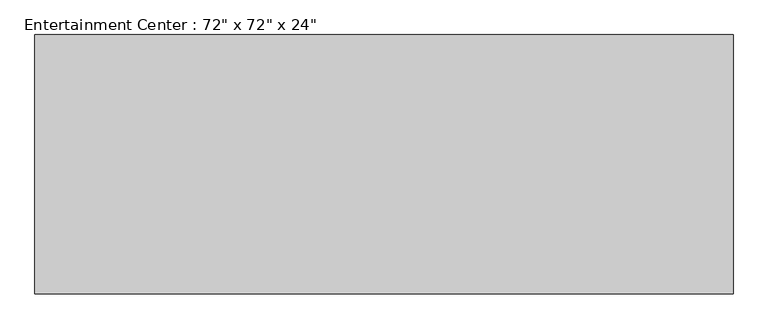
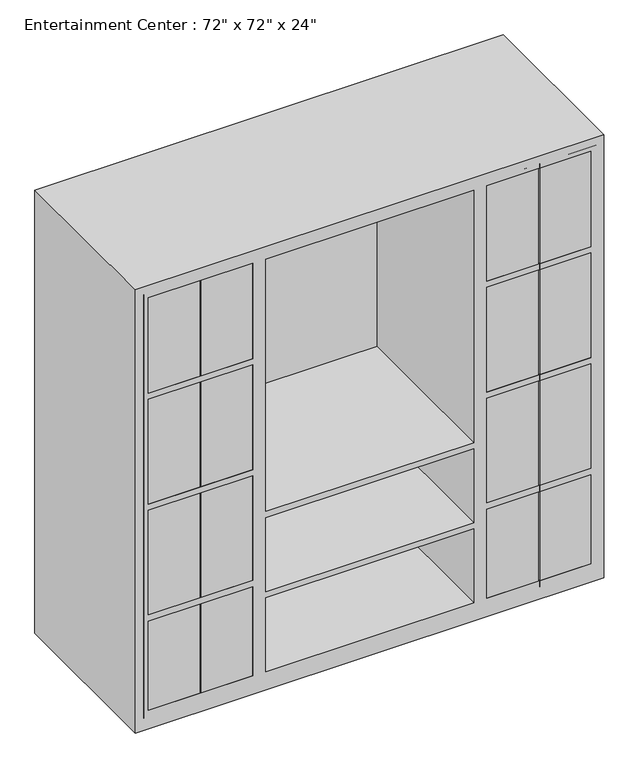
"""IFC4 building model written with IfcOpenShell, lengths in millimetres: furniture geometry."""

from ifc_helpers import new_model, si_unit, point, frame, frame_2d, origin, place, context, project, spatial, polyline, circle_curve, trimmed, segment, composite_curve, outline, extrude, faceted_brep, source, transform, mapped, element, save


def furniture_cf0b6580(model_context):
    return source(origin(), model_context, "Body", "SolidModel", [
        faceted_brep([(914.4, -781.05, 0.0), (914.4, -781.05, 1828.8), (-914.4, -781.05, 1828.8), (-914.4, -781.05, 0.0), (-457.2, -781.05, 1778.0), (-457.2, -781.05, 1384.3), (-863.6, -781.05, 1384.3), (-863.6, -781.05, 1778.0), (-457.2, -781.05, 76.2), (-863.6, -781.05, 76.2), (-863.6, -781.05, 444.5), (-457.2, -781.05, 444.5), (863.6, -781.05, 1384.3), (457.2, -781.05, 1384.3), (457.2, -781.05, 1778.0), (863.6, -781.05, 1778.0), (-406.4, -781.05, 736.6), (-406.4, -781.05, 1778.0), (406.4, -781.05, 1778.0), (406.4, -781.05, 736.6), (406.4, -781.05, 76.2), (-406.4, -781.05, 76.2), (-406.4, -781.05, 381.0), (406.4, -781.05, 381.0), (863.6, -781.05, 76.2), (457.2, -781.05, 76.2), (457.2, -781.05, 444.5), (863.6, -781.05, 444.5), (-863.6, -781.05, 469.9), (-863.6, -781.05, 901.7), (-457.2, -781.05, 901.7), (-457.2, -781.05, 469.9), (-457.2, -781.05, 1358.9), (-457.2, -781.05, 927.1), (-863.6, -781.05, 927.1), (-863.6, -781.05, 1358.9), (457.2, -781.05, 1358.9), (863.6, -781.05, 1358.9), (863.6, -781.05, 927.1), (457.2, -781.05, 927.1), (457.2, -781.05, 901.7), (863.6, -781.05, 901.7), (863.6, -781.05, 469.9), (457.2, -781.05, 469.9), (406.4, -781.05, 406.4), (-406.4, -781.05, 406.4), (-406.4, -781.05, 711.2), (406.4, -781.05, 711.2), (914.4, -101.6, 0.0), (-914.4, -101.6, 0.0), (-914.4, -101.6, 1828.8), (914.4, -101.6, 1828.8), (-457.2, -127.0, 1778.0), (-457.2, -127.0, 1384.3), (-863.6, -127.0, 1384.3), (-863.6, -127.0, 1778.0), (-457.2, -127.0, 76.2), (-863.6, -127.0, 76.2), (-863.6, -127.0, 444.5), (-457.2, -127.0, 444.5), (863.6, -127.0, 1384.3), (457.2, -127.0, 1384.3), (457.2, -127.0, 1778.0), (863.6, -127.0, 1778.0), (-406.4, -127.0, 736.6), (-406.4, -127.0, 1778.0), (406.4, -127.0, 1778.0), (406.4, -127.0, 736.6), (406.4, -127.0, 76.2), (-406.4, -127.0, 76.2), (-406.4, -127.0, 381.0), (406.4, -127.0, 381.0), (863.6, -127.0, 76.2), (457.2, -127.0, 76.2), (457.2, -127.0, 444.5), (863.6, -127.0, 444.5), (-863.6, -127.0, 469.9), (-863.6, -127.0, 901.7), (-457.2, -127.0, 901.7), (-457.2, -127.0, 469.9), (-457.2, -127.0, 1358.9), (-457.2, -127.0, 927.1), (-863.6, -127.0, 927.1), (-863.6, -127.0, 1358.9), (457.2, -127.0, 1358.9), (863.6, -127.0, 1358.9), (863.6, -127.0, 927.1), (457.2, -127.0, 927.1), (457.2, -127.0, 901.7), (863.6, -127.0, 901.7), (863.6, -127.0, 469.9), (457.2, -127.0, 469.9), (406.4, -127.0, 406.4), (-406.4, -127.0, 406.4), (-406.4, -127.0, 711.2), (406.4, -127.0, 711.2)], [[[0, 1, 2, 3], [4, 5, 6, 7], [8, 9, 10, 11], [12, 13, 14, 15], [16, 17, 18, 19], [20, 21, 22, 23], [24, 25, 26, 27], [28, 29, 30, 31], [32, 33, 34, 35], [36, 37, 38, 39], [40, 41, 42, 43], [44, 45, 46, 47]], [[48, 49, 50, 51]], [[1, 0, 48, 51]], [[2, 1, 51, 50]], [[3, 2, 50, 49]], [[0, 3, 49, 48]], [[5, 4, 52, 53]], [[6, 5, 53, 54]], [[7, 6, 54, 55]], [[4, 7, 55, 52]], [[9, 8, 56, 57]], [[10, 9, 57, 58]], [[11, 10, 58, 59]], [[8, 11, 59, 56]], [[13, 12, 60, 61]], [[14, 13, 61, 62]], [[15, 14, 62, 63]], [[12, 15, 63, 60]], [[17, 16, 64, 65]], [[18, 17, 65, 66]], [[19, 18, 66, 67]], [[16, 19, 67, 64]], [[21, 20, 68, 69]], [[22, 21, 69, 70]], [[23, 22, 70, 71]], [[20, 23, 71, 68]], [[25, 24, 72, 73]], [[26, 25, 73, 74]], [[27, 26, 74, 75]], [[24, 27, 75, 72]], [[29, 28, 76, 77]], [[30, 29, 77, 78]], [[31, 30, 78, 79]], [[28, 31, 79, 76]], [[33, 32, 80, 81]], [[34, 33, 81, 82]], [[35, 34, 82, 83]], [[32, 35, 83, 80]], [[37, 36, 84, 85]], [[38, 37, 85, 86]], [[39, 38, 86, 87]], [[36, 39, 87, 84]], [[41, 40, 88, 89]], [[42, 41, 89, 90]], [[43, 42, 90, 91]], [[40, 43, 91, 88]], [[45, 44, 92, 93]], [[46, 45, 93, 94]], [[47, 46, 94, 95]], [[44, 47, 95, 92]], [[53, 52, 55, 54]], [[57, 56, 59, 58]], [[61, 60, 63, 62]], [[65, 64, 67, 66]], [[69, 68, 71, 70]], [[73, 72, 75, 74]], [[77, 76, 79, 78]], [[81, 80, 83, 82]], [[85, 84, 87, 86]], [[89, 88, 91, 90]], [[93, 92, 95, 94]]]),
        extrude(outline(composite_curve([segment(polyline([(1003.3, -632.9986452), (1003.3, -657.225), (825.5, -657.225), (825.5, -632.9986452)]), True, "CONTINUOUS"), segment(trimmed(circle_curve(frame_2d((850.9, -632.9986452)), 25.4), [point((825.5, -632.9986452))], [point((850.9, -607.5986452))], False, "CARTESIAN"), True, "CONTINUOUS"), segment(polyline([(850.9, -607.5986452), (977.9, -607.5986452)]), True, "CONTINUOUS"), segment(trimmed(circle_curve(frame_2d((977.9, -632.9986452)), 25.4), [point((977.9, -607.5986452))], [point((1003.3, -632.9986452))], False, "CARTESIAN"), True, "CONTINUOUS")], self_intersect=False)), frame((0.0, -714.375, 0.0), z_axis=(0.0, 1.0, 0.0), x_axis=(0.0, 0.0, 1.0)), (0.0, 0.0, 1.0), 3.175),
        extrude(outline(composite_curve([segment(trimmed(circle_curve(frame_2d((977.9, -688.18125)), 25.4), [point((1003.3, -688.18125))], [point((977.9, -713.58125))], False, "CARTESIAN"), True, "CONTINUOUS"), segment(polyline([(977.9, -713.58125), (850.9, -713.58125)]), True, "CONTINUOUS"), segment(trimmed(circle_curve(frame_2d((850.9, -688.18125)), 25.4), [point((850.9, -713.58125))], [point((825.5, -688.18125))], False, "CARTESIAN"), True, "CONTINUOUS"), segment(polyline([(825.5, -688.18125), (825.5, -663.575), (1003.3, -663.575), (1003.3, -688.18125)]), True, "CONTINUOUS")], self_intersect=False)), frame((0.0, -714.375, 0.0), z_axis=(0.0, 1.0, 0.0), x_axis=(0.0, 0.0, 1.0)), (0.0, 0.0, 1.0), 3.175),
        extrude(outline(composite_curve([segment(trimmed(circle_curve(frame_2d((977.9, 632.9986452)), 25.4), [point((1003.3, 632.9986452))], [point((977.9, 607.5986452))], False, "CARTESIAN"), True, "CONTINUOUS"), segment(polyline([(977.9, 607.5986452), (850.9, 607.5986452)]), True, "CONTINUOUS"), segment(trimmed(circle_curve(frame_2d((850.9, 632.9986452)), 25.4), [point((850.9, 607.5986452))], [point((825.5, 632.9986452))], False, "CARTESIAN"), True, "CONTINUOUS"), segment(polyline([(825.5, 632.9986452), (825.5, 657.225), (1003.3, 657.225), (1003.3, 632.9986452)]), True, "CONTINUOUS")], self_intersect=False)), frame((0.0, -714.375, 0.0), z_axis=(0.0, 1.0, 0.0), x_axis=(0.0, 0.0, 1.0)), (0.0, 0.0, 1.0), 3.175),
        extrude(outline(composite_curve([segment(polyline([(1003.3, 688.18125), (1003.3, 663.575), (825.5, 663.575), (825.5, 688.18125)]), True, "CONTINUOUS"), segment(trimmed(circle_curve(frame_2d((850.9, 688.18125)), 25.4), [point((825.5, 688.18125))], [point((850.9, 713.58125))], False, "CARTESIAN"), True, "CONTINUOUS"), segment(polyline([(850.9, 713.58125), (977.9, 713.58125)]), True, "CONTINUOUS"), segment(trimmed(circle_curve(frame_2d((977.9, 688.18125)), 25.4), [point((977.9, 713.58125))], [point((1003.3, 688.18125))], False, "CARTESIAN"), True, "CONTINUOUS")], self_intersect=False)), frame((0.0, -714.375, 0.0), z_axis=(0.0, 1.0, 0.0), x_axis=(0.0, 0.0, 1.0)), (0.0, 0.0, 1.0), 3.175),
        extrude(outline(polyline([(-882.65, -711.2), (-663.575, -711.2), (-663.575, -781.05), (-882.65, -781.05), (-882.65, -711.2)])), frame((0.0, 0.0, 50.8), z_axis=(0.0, 0.0, 1.0), x_axis=(1.0, 0.0, 0.0)), (0.0, 0.0, 1.0), 1746.25),
        extrude(outline(polyline([(-657.225, -711.2), (-438.15, -711.2), (-438.15, -781.05), (-657.225, -781.05), (-657.225, -711.2)])), frame((0.0, 0.0, 50.8), z_axis=(0.0, 0.0, 1.0), x_axis=(1.0, 0.0, 0.0)), (0.0, 0.0, 1.0), 1746.25),
        extrude(outline(polyline([(663.575, -711.2), (882.65, -711.2), (882.65, -781.05), (663.575, -781.05), (663.575, -711.2)])), frame((0.0, 0.0, 50.8), z_axis=(0.0, 0.0, 1.0), x_axis=(1.0, 0.0, 0.0)), (0.0, 0.0, 1.0), 1746.25),
        extrude(outline(polyline([(438.15, -711.2), (657.225, -711.2), (657.225, -781.05), (438.15, -781.05), (438.15, -711.2)])), frame((0.0, 0.0, 50.8), z_axis=(0.0, 0.0, 1.0), x_axis=(1.0, 0.0, 0.0)), (0.0, 0.0, 1.0), 1746.25),
    ])


if __name__ == "__main__":
    model = new_model("IFC4")
    model_context = context("Model", 3, world=origin())
    ifc_project = project(units=[si_unit("LENGTHUNIT", "METRE", prefix="MILLI")], contexts=[model_context])
    site = spatial("IfcSite", under=ifc_project)
    building = spatial("IfcBuilding", under=site)
    placement = place(None, origin())
    furniture_shape = furniture_cf0b6580(model_context)
    element("IfcFurniture", 1, ObjectType="Entertainment Center : 72\" x 72\" x 24\"", at=placement, inside=building, context=model_context, shape_type="MappedRepresentation", body=[
        mapped(furniture_shape, transform((0.0, 0.0, 0.0), x_axis=(1.0, 0.0, 0.0), y_axis=(0.0, 1.0, 0.0), z_axis=(0.0, 0.0, 1.0))),
    ])
    save(model, "model.ifc")

# Revit data of these elements
# Type "Entertainment Center : 72\" x 72\" x 24\""
#   Assembly Code = "E2020200"
#   Center Width = 2' - 8"
#   Depth = 2' - 0"
#   Height = 6' - 0"
#   Width = 6' - 0"
#   Material = Wood
#   Default Elevation = 0
# Element 1 (IfcFurniture, "Entertainment Center : 72\" x 72\" x 24\"")
#   Materials on its faces: "Wood", "Steel, Chrome Plated", "Glass - Clear, Grey"
# Materials
#   "Wood": class "Wood", colour RGB 0 0 0, transparency 0, Description = "Generic wood", Cost = 0
#   "Steel, Chrome Plated": class "Metal", colour RGB 17 17 17, transparency 0, Description = "Chromiuim plated steel", Cost = 0
#   "Glass - Clear, Grey": class "Glass", colour RGB 252 255 255, transparency 0.64
